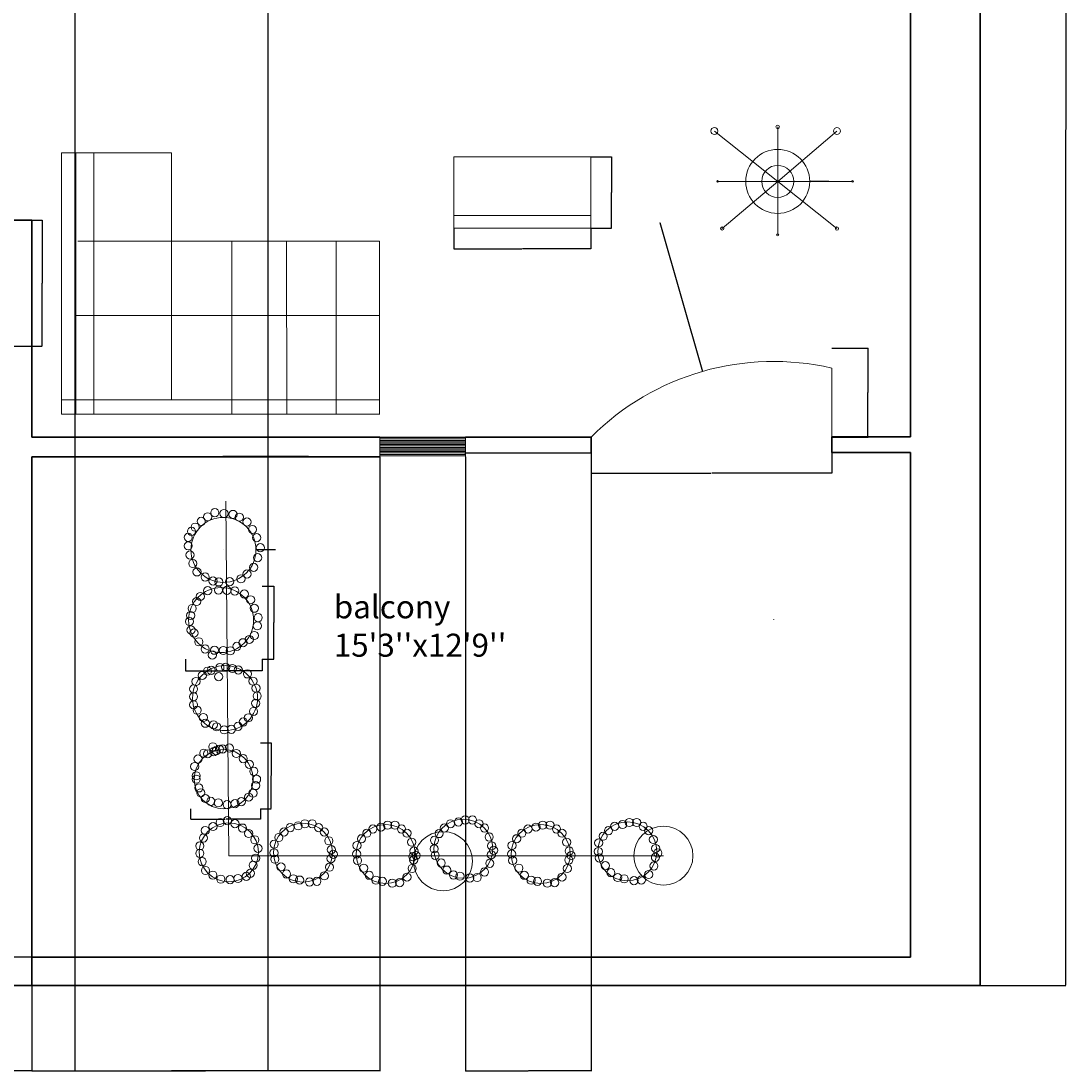
# Model space of a CAD drawing. Units: millimetres. Extents: x 1942 to 12281, y -2698 to 3078.
# Tile 5 of 6: x 9104 to 12281, y -2646 to 547. Entities that reach past the tile are written whole.
import ezdxf

# ---------------------------------------------------------------- set-up
doc = ezdxf.new("R2010")
doc.units = ezdxf.units.MM
for name, color, linetype, lineweight in [('A-ANNO-DIMS', 2, 'Continuous', 18), ('A-AREA-IDEN', 3, 'Continuous', 18), ('A-DOOR', 4, 'Continuous', 18), ('A-FURN', 8, 'Continuous', 18), ('A-GLAZ', 4, 'Continuous', 18), ('A-GLAZ-PATT', 9, 'Continuous', 13), ('A-WALL', 7, 'Continuous', 35), ('E-LITE', 6, 'Continuous', 18), ('L-PLNT', 3, 'Continuous', 13)]:
    doc.layers.add(name, color=color, linetype=linetype, lineweight=lineweight)
doc.styles.get("Standard").update_dxf_attribs({"font": 'arial.ttf'})
doc.dimstyles.get("Standard").update_dxf_attribs({"dimtxt": 0.18, "dimasz": 0.18, "dimexe": 0.18, "dimexo": 0.0625, "dimgap": 0.09, "dimtad": 0, "dimtih": 1, "dimtoh": 1, "dimdec": 4, "dimzin": 0, "dimdsep": 46, "dimtxsty": 'Standard', "dimcen": 0.09, "dimadec": 0, "dimazin": 0, "dimtfac": 1, "dimtdec": 4, "dimtofl": 0, "dimtmove": 0, "dimatfit": 3, "dimfxl": 1, "dimtolj": 1, "dimtzin": 0, "dimarcsym": 0})

# ---------------------------------------------------------------- blocks, each defined once
blk = doc.blocks.new('SOFA-SECTIONAL')
for p, q in [((0, 794.3), (0, 0)), ((0, 794.3), (334.4, 794.3)), ((43.6, 794.3), (43.6, 0)), ((98.1, 794.3), (98.1, 0)), ((334.4, 794.3), (334.4, 43.6)), ((49.7, 525.6), (966.1, 525.6)), ((517.7, 525.6), (517.9, 0)), ((684.1, 525.6), (684.3, 0)), ((834.9, 525.6), (835.1, 0)), ((966.1, 525.6), (966.3, 0)), ((43.6, 299.6), (966.2, 299.6)), ((0, 43.6), (967.4, 43.6)), ((0, 0), (967.4, 0))]:
    blk.add_line(p, q)
blk = doc.blocks.new('SEAT-LIVING')
for p, q in [((0, 38.6), (0, 0)), ((416.9, 0), (416.9, 38.6)), ((0, 0), (416.9, 0))]:
    blk.add_line(p, q)
blk.add_lwpolyline([(0, 217.2), (416.9, 217.2), (416.9, 38.6), (0, 38.6)], close=True)
blk = doc.blocks.new('CHANDELIER-8ARM')
for p, q in [((203.2, 166), (203.2, 331.7)), ((10.7, 319.2), (10.7, 319.2)), ((203.2, 166), (10.7, 319.2)), ((203.2, 166), (383.4, 319.2)), ((203.2, 166), (20.4, 166)), ((203.2, 166), (34.5, 22.7)), ((203.2, 166), (430.7, 166)), ((203.2, 166), (203.2, 3.4)), ((203.2, 166), (383.4, 22.7))]:
    blk.add_line(p, q)
for centre, radius in [((10.7, 319.2), 10.7), ((203.2, 331.7), 5.5), ((383.4, 319.2), 10.2), ((203.2, 166), 97.3), ((203.2, 166), 97.3), ((203.2, 166), 48.7), ((20.4, 166), 2.45), ((430.7, 166), 2.45), ((34.5, 22.7), 4.8), ((203.2, 3.4), 3.36), ((383.4, 22.7), 4.98)]:
    blk.add_circle(centre, radius)
blk = doc.blocks.new('DOOR-ENTRY')
blk.add_line((731.8, 0.7), (731.8, 209.8))
blk.add_arc((555.2, -555.3), 785.2, 77.0012, 134.997)
blk = doc.blocks.new('PLANT-ROUND')
for centre, radius in [((86.1, 183), 12.4), ((106.4, 189), 12.4), ((128.8, 189), 12.4), ((100.7, 101.4), 89.7), ((27.3, 147.6), 12.4), ((43.2, 164.4), 12.4), ((61.8, 177.4), 12.4), ((148.6, 177.4), 12.4), ((165.4, 164.4), 12.4), ((13.3, 127.1), 12.4), ((179.4, 137.3), 12.4), ((12.4, 101), 12.4), ((186.9, 110.3), 12.4), ((193.1, 96.5), 12.4), ((15.2, 81.4), 12.4), ((33.8, 58.1), 12.4), ((181.3, 57.1), 12.4), ((185.9, 83.2), 12.4), ((50.6, 36.6), 12.4), ((71.2, 21.7), 12.4), ((165.4, 31), 12.4), ((90.8, 18), 12.4), ((120.6, 12.4), 12.4), ((143, 14.2), 12.4)]:
    blk.add_circle(centre, radius)
blk = doc.blocks.new('PLANT-ROUND-2')
for centre, radius in [((93.4, 223.1), 12.4), ((121.1, 220.4), 12.4), ((148.7, 217.6), 12.4), ((119.6, 109.8), 98.8), ((52, 196.4), 12.4), ((71.3, 210.2), 12.4), ((168, 209.3), 12.4), ((191, 194.6), 12.4), ((12.4, 147.7), 12.4), ((22.5, 166.1), 12.4), ((33.6, 178.9), 12.4), ((207.6, 171.6), 12.4), ((12.4, 121.9), 12.4), ((220.5, 146.7), 12.4), ((231.6, 116.4), 12.4), ((17.9, 94.3), 12.4), ((223.3, 86), 12.4), ((26.2, 68.5), 12.4), ((211.3, 56.6), 12.4), ((39.1, 42.8), 12.4), ((64, 27.1), 12.4), ((172.6, 21.6), 12.4), ((191, 36.3), 12.4), ((87.9, 15.1), 12.4), ((105.4, 12.4), 12.4), ((138.6, 13.3), 12.4)]:
    blk.add_circle(centre, radius)
blk = doc.blocks.new('PLANT-ROUND-3')
for centre, radius in [((108.8, 118.6), 98.8), ((45.5, 190.7), 12.4), ((67.6, 208.2), 12.4), ((100.8, 210), 12.4), ((126.6, 209.1), 12.4), ((150.5, 207.3), 12.4), ((179.1, 198.1), 12.4), ((198.4, 180.6), 12.4), ((20.7, 153.9), 12.4), ((34.5, 175.1), 12.4), ((209.5, 154.8), 12.4), ((16.1, 132.7), 12.4), ((221.4, 126.3), 12.4), ((12.4, 114.3), 12.4), ((17, 88.6), 12.4), ((218.7, 101.4), 12.4), ((26.2, 79.4), 12.4), ((40.9, 52.7), 12.4), ((194.7, 60), 12.4), ((209.5, 72), 12.4), ((60.1, 30.8), 12.4), ((88.6, 27.1), 12.4), ((115.3, 26.2), 12.4), ((136.5, 25.3), 12.4), ((156.7, 39.1), 12.4), ((175.4, 49.9), 12.4), ((82.2, 12.4), 12.4), ((82.2, 12.4), 12.4), ((82.2, 12.4), 12.4)]:
    blk.add_circle(centre, radius)
blk = doc.blocks.new('PLANT-ROUND-4')
for centre, radius in [((108, 108.9), 98.8), ((54.7, 190.9), 12.4), ((65.8, 193.7), 12.4), ((92.5, 202), 12.4), ((110, 202.9), 12.4), ((130.3, 199.2), 12.4), ((148.7, 194.6), 12.4), ((176.3, 182.6), 12.4), ((19.8, 159.6), 12.4), ((39.1, 178), 12.4), ((88.8, 174.3), 12.4), ((88.8, 174.3), 12.4), ((88.8, 174.3), 12.4), ((88.8, 174.3), 12.4), ((192.9, 160.5), 12.4), ((12.4, 136.6), 12.4), ((202.1, 139.4), 12.4), ((205.8, 115.5), 12.4), ((12.4, 113.6), 12.4), ((12.4, 88.8), 12.4), ((201.2, 93.4), 12.4), ((23.4, 72.2), 12.4), ((194.7, 68.5), 12.4), ((41.9, 50.1), 12.4), ((48.3, 32.6), 12.4), ((73.2, 28), 12.4), ((82.4, 21.6), 12.4), ((147.8, 23.4), 12.4), ((163.4, 36.3), 12.4), ((179.1, 49.2), 12.4), ((105.4, 12.4), 12.4), ((127.5, 14.2), 12.4)]:
    blk.add_circle(centre, radius)
blk = doc.blocks.new('PLANT-ROUND-5')
for centre, radius in [((67.6, 188.1), 12.4), ((87.9, 180.8), 12.4), ((97.1, 181.7), 12.4), ((117.6, 184.4), 12.4), ((22.5, 151.3), 12.4), ((100.5, 89.8), 89.7), ((40, 168.8), 12.4), ((52, 167), 12.4), ((70.4, 173.4), 12.4), ((77.8, 176.2), 12.4), ((138.8, 167.8), 12.4), ((159.9, 152.2), 12.4), ((12.4, 128.3), 12.4), ((178.4, 134.7), 12.4), ((17, 99.8), 12.4), ((17, 89.7), 12.4), ((192.2, 113.5), 12.4), ((200.5, 89.6), 12.4), ((25, 63.2), 12.4), ((25, 63.2), 12.4), ((25, 63.2), 12.4), ((25, 63.2), 12.4), ((25, 63.2), 12.4), ((25, 63.2), 12.4), ((197.7, 70.3), 12.4), ((30.8, 48.3), 12.4), ((44.6, 30.8), 12.4), ((61.2, 22.5), 12.4), ((154.2, 21.6), 12.4), ((176.5, 35.3), 12.4), ((189.4, 47.2), 12.4), ((84.2, 17.9), 12.4), ((110.9, 12.4), 12.4), ((134.9, 15.1), 12.4)]:
    blk.add_circle(centre, radius)
blk = doc.blocks.new('PLANT-ROUND-6')
for centre, radius in [((74, 186.3), 12.4), ((95.8, 192.1), 12.4), ((119.1, 182.8), 12.4), ((100.5, 95.9), 89.7), ((28.8, 162.1), 12.4), ((52.4, 174), 12.4), ((141.9, 169.4), 12.4), ((160.8, 153), 12.4), ((23.3, 139.1), 12.4), ((179.6, 133.8), 12.4), ((12.4, 115.2), 12.4), ((12.4, 92.5), 12.4), ((189.2, 107.7), 12.4), ((19.4, 67.4), 12.4), ((174.3, 56.2), 12.4), ((182.2, 78), 12.4), ((29.6, 40.4), 12.4), ((52, 26.4), 12.4), ((153.8, 22.6), 12.4), ((165.9, 32), 12.4), ((76.3, 14.2), 12.4), ((104.3, 12.4), 12.4), ((128.6, 16.1), 12.4)]:
    blk.add_circle(centre, radius)
blk = doc.blocks.new('WIN-LIVING')
for p, q in [((0, 59.6), (0, 0)), ((0, 59.6), (260.2, 59.6)), ((260.2, 0), (260.2, 59.6))]:
    blk.add_line(p, q)
blk = doc.blocks.new('*D30')
at = {"layer": 'A-ANNO-DIMS', "color": 0, "lineweight": -2, "transparency": 16777216}
for p, q in [((10419.7, -83.7), (10419.7, -146.3)), ((10836.6, -83.7), (10836.6, -146.3)), ((10419.9, -146.2), (10627.2, -146.2)), ((10836.4, -146.2), (10629.1, -146.2))]:
    blk.add_line(p, q, dxfattribs=at)
at = {"layer": 'A-ANNO-DIMS', "color": 0, "transparency": 16777216}
for points in [[(10419.9, -146.1), (10419.9, -146.2), (10419.7, -146.2)], [(10836.4, -146.1), (10836.4, -146.2), (10836.6, -146.2)]]:
    blk.add_solid(points, dxfattribs=at)
at = {"layer": 'Defpoints', "color": 0, "transparency": 16777216}
for p in [(10419.7, -83.6), (10836.6, -83.6), (10836.6, -146.2)]:
    blk.add_point(p, dxfattribs=at)
at = {"layer": 'A-ANNO-DIMS', "color": 0, "transparency": 16777216, "insert": (10628.2, -146.2), "char_height": 0.18, "attachment_point": 5}
blk.add_mtext('\\A1;SEAT 417 TYP.', dxfattribs=at)
blk = doc.blocks.new('*D31')
at = {"layer": 'A-ANNO-DIMS', "color": 0, "lineweight": -2, "transparency": 16777216}
for p, q in [((10836.7, 133.5), (10899.3, 133.5)), ((10899.1, 133.4), (10899.1, 25.1)), ((10899.1, -83.4), (10899.1, 24.8)), ((10836.7, -83.6), (10899.3, -83.6))]:
    blk.add_line(p, q, dxfattribs=at)
at = {"layer": 'A-ANNO-DIMS', "color": 0, "transparency": 16777216}
for points in [[(10899.1, 133.4), (10899.2, 133.4), (10899.1, 133.5)], [(10899.1, -83.4), (10899.2, -83.4), (10899.1, -83.6)]]:
    blk.add_solid(points, dxfattribs=at)
at = {"layer": 'Defpoints', "color": 0, "transparency": 16777216}
for p in [(10836.6, 133.5), (10899.1, 133.5), (10836.6, -83.6)]:
    blk.add_point(p, dxfattribs=at)
at = {"layer": 'A-ANNO-DIMS', "color": 0, "transparency": 16777216, "insert": (10899.1, 25), "char_height": 0.18, "attachment_point": 5}
blk.add_mtext('\\A1;217 TYP.', dxfattribs=at)
blk = doc.blocks.new('*D39')
at = {"layer": 'A-ANNO-DIMS', "color": 0, "lineweight": -2, "transparency": 16777216}
for p, q in [((9071.9, -58.9), (9169.3, -58.9)), ((9169.1, -59), (9169.1, -250.1)), ((9169.1, -441.5), (9169.1, -250.5)), ((9071.9, -441.7), (9169.3, -441.7))]:
    blk.add_line(p, q, dxfattribs=at)
at = {"layer": 'A-ANNO-DIMS', "color": 0, "transparency": 16777216}
for points in [[(9169.1, -59), (9169.1, -59), (9169.1, -58.9)], [(9169.1, -441.5), (9169.1, -441.5), (9169.1, -441.7)]]:
    blk.add_solid(points, dxfattribs=at)
at = {"layer": 'Defpoints', "color": 0, "transparency": 16777216}
for p in [(9071.8, -58.9), (9169.1, -58.9), (9071.8, -441.7)]:
    blk.add_point(p, dxfattribs=at)
at = {"layer": 'A-ANNO-DIMS', "color": 0, "transparency": 16777216, "insert": (9169.1, -250.3), "char_height": 0.18, "attachment_point": 5}
blk.add_mtext('\\A1;383 TYP.', dxfattribs=at)
blk = doc.blocks.new('*D40')
at = {"layer": 'A-ANNO-DIMS', "color": 0, "lineweight": -2, "transparency": 16777216}
for p, q in [((10837.4, -718.5), (10837.4, -828.4)), ((11569.2, -718.5), (11569.2, -828.4)), ((10837.5, -828.2), (11201.8, -828.2)), ((11569, -828.2), (11204.7, -828.2))]:
    blk.add_line(p, q, dxfattribs=at)
at = {"layer": 'A-ANNO-DIMS', "color": 0, "transparency": 16777216}
for points in [[(10837.5, -828.1), (10837.5, -828.2), (10837.4, -828.2)], [(11569, -828.1), (11569, -828.2), (11569.2, -828.2)]]:
    blk.add_solid(points, dxfattribs=at)
at = {"layer": 'Defpoints', "color": 0, "transparency": 16777216}
for p in [(10837.4, -718.4), (11569.2, -718.4), (11569.2, -828.2)]:
    blk.add_point(p, dxfattribs=at)
at = {"layer": 'A-ANNO-DIMS', "color": 0, "transparency": 16777216, "insert": (11203.3, -828.2), "char_height": 0.18, "attachment_point": 5}
blk.add_mtext('\\A1;ENTRY DOOR 732 TYP.', dxfattribs=at)
blk = doc.blocks.new('*D41')
at = {"layer": 'A-ANNO-DIMS', "color": 0, "lineweight": -2, "transparency": 16777216}
for p, q in [((11569.3, -447.7), (11679.2, -447.7)), ((11679, -447.8), (11679, -582.8)), ((11679, -718.2), (11679, -583.2)), ((11569.3, -718.4), (11679.2, -718.4))]:
    blk.add_line(p, q, dxfattribs=at)
at = {"layer": 'A-ANNO-DIMS', "color": 0, "transparency": 16777216}
for points in [[(11678.9, -447.8), (11679, -447.8), (11679, -447.7)], [(11678.9, -718.2), (11679, -718.2), (11679, -718.4)]]:
    blk.add_solid(points, dxfattribs=at)
at = {"layer": 'Defpoints', "color": 0, "transparency": 16777216}
for p in [(11569.2, -447.7), (11679, -447.7), (11569.2, -718.4)]:
    blk.add_point(p, dxfattribs=at)
at = {"layer": 'A-ANNO-DIMS', "color": 0, "transparency": 16777216, "insert": (11679, -583), "char_height": 0.18, "attachment_point": 5}
blk.add_mtext('\\A1;271 TYP.', dxfattribs=at)
blk = doc.blocks.new('*D52')
at = {"layer": 'A-ANNO-DIMS', "color": 0, "lineweight": -2, "transparency": 16777216}
for p, q in [((9604.1, -1393.8), (9604.1, -1429)), ((9837.9, -1393.8), (9837.9, -1429)), ((9604.3, -1428.8), (9719.8, -1428.8)), ((9837.7, -1428.8), (9722.2, -1428.8))]:
    blk.add_line(p, q, dxfattribs=at)
at = {"layer": 'A-ANNO-DIMS', "color": 0, "transparency": 16777216}
for points in [[(9604.3, -1428.8), (9604.3, -1428.8), (9604.1, -1428.8)], [(9837.7, -1428.8), (9837.7, -1428.8), (9837.9, -1428.8)]]:
    blk.add_solid(points, dxfattribs=at)
at = {"layer": 'Defpoints', "color": 0, "transparency": 16777216}
for p in [(9604.1, -1393.7), (9837.9, -1393.7), (9837.9, -1428.8)]:
    blk.add_point(p, dxfattribs=at)
at = {"layer": 'A-ANNO-DIMS', "color": 0, "transparency": 16777216, "insert": (9721, -1428.8), "char_height": 0.18, "attachment_point": 5}
blk.add_mtext('\\A1;PLANT C 234 TYP.', dxfattribs=at)
blk = doc.blocks.new('*D53')
at = {"layer": 'A-ANNO-DIMS', "color": 0, "lineweight": -2, "transparency": 16777216}
for p, q in [((9838, -1171.3), (9873.2, -1171.3)), ((9873, -1171.5), (9873, -1282.3)), ((9873, -1393.5), (9873, -1282.7)), ((9838, -1393.7), (9873.2, -1393.7))]:
    blk.add_line(p, q, dxfattribs=at)
at = {"layer": 'A-ANNO-DIMS', "color": 0, "transparency": 16777216}
for points in [[(9872.9, -1171.5), (9873, -1171.5), (9873, -1171.3)], [(9872.9, -1393.5), (9873, -1393.5), (9873, -1393.7)]]:
    blk.add_solid(points, dxfattribs=at)
at = {"layer": 'Defpoints', "color": 0, "transparency": 16777216}
for p in [(9837.9, -1171.3), (9873, -1171.3), (9837.9, -1393.7)]:
    blk.add_point(p, dxfattribs=at)
at = {"layer": 'A-ANNO-DIMS', "color": 0, "transparency": 16777216, "insert": (9873, -1282.5), "char_height": 0.18, "attachment_point": 5}
blk.add_mtext('\\A1;222 TYP.', dxfattribs=at)
blk = doc.blocks.new('*D56')
at = {"layer": 'A-ANNO-DIMS', "color": 0, "lineweight": -2, "transparency": 16777216}
for p, q in [((9620.1, -1848.4), (9620.1, -1880.5)), ((9833, -1848.4), (9833, -1880.5)), ((9620.3, -1880.3), (9725.4, -1880.3)), ((9832.8, -1880.3), (9727.7, -1880.3))]:
    blk.add_line(p, q, dxfattribs=at)
at = {"layer": 'A-ANNO-DIMS', "color": 0, "transparency": 16777216}
for points in [[(9620.3, -1880.3), (9620.3, -1880.3), (9620.1, -1880.3)], [(9832.8, -1880.3), (9832.8, -1880.3), (9833, -1880.3)]]:
    blk.add_solid(points, dxfattribs=at)
at = {"layer": 'Defpoints', "color": 0, "transparency": 16777216}
for p in [(9620.1, -1848.4), (9833, -1848.4), (9833, -1880.3)]:
    blk.add_point(p, dxfattribs=at)
at = {"layer": 'A-ANNO-DIMS', "color": 0, "transparency": 16777216, "insert": (9726.5, -1880.3), "char_height": 0.18, "attachment_point": 5}
blk.add_mtext('\\A1;PLANT E 213 TYP.', dxfattribs=at)
blk = doc.blocks.new('*D57')
at = {"layer": 'A-ANNO-DIMS', "color": 0, "lineweight": -2, "transparency": 16777216}
for p, q in [((9833, -1647.8), (9865.1, -1647.8)), ((9864.9, -1648), (9864.9, -1747.9)), ((9864.9, -1848.2), (9864.9, -1748.3)), ((9833, -1848.4), (9865.1, -1848.4))]:
    blk.add_line(p, q, dxfattribs=at)
at = {"layer": 'A-ANNO-DIMS', "color": 0, "transparency": 16777216}
for points in [[(9864.9, -1648), (9864.9, -1648), (9864.9, -1647.8)], [(9864.9, -1848.2), (9864.9, -1848.2), (9864.9, -1848.4)]]:
    blk.add_solid(points, dxfattribs=at)
at = {"layer": 'Defpoints', "color": 0, "transparency": 16777216}
for p in [(9833, -1647.8), (9864.9, -1647.8), (9833, -1848.4)]:
    blk.add_point(p, dxfattribs=at)
at = {"layer": 'A-ANNO-DIMS', "color": 0, "transparency": 16777216, "insert": (9864.9, -1748.1), "char_height": 0.18, "attachment_point": 5}
blk.add_mtext('\\A1;201 TYP.', dxfattribs=at)
blk = doc.blocks.new('*D93')
at = {"layer": 'A-ANNO-DIMS', "color": 0, "lineweight": -2, "transparency": 16777216}
for p, q in [((12020.6, 2817.6), (12281, 2817.6)), ((12280.8, 2817.4), (12280.8, 216.2)), ((12280.8, -2385.3), (12280.8, 215.9)), ((12020.6, -2385.5), (12281, -2385.5))]:
    blk.add_line(p, q, dxfattribs=at)
at = {"layer": 'A-ANNO-DIMS', "color": 0, "transparency": 16777216}
for points in [[(12280.7, 2817.4), (12280.8, 2817.4), (12280.8, 2817.6)], [(12280.7, -2385.3), (12280.8, -2385.3), (12280.8, -2385.5)]]:
    blk.add_solid(points, dxfattribs=at)
at = {"layer": 'Defpoints', "color": 0, "transparency": 16777216}
for p in [(12020.6, 2817.6), (12280.8, 2817.6), (12020.6, -2385.5)]:
    blk.add_point(p, dxfattribs=at)
at = {"layer": 'A-ANNO-DIMS', "color": 0, "transparency": 16777216, "insert": (12280.8, 216.1), "char_height": 0.18, "attachment_point": 5}
blk.add_mtext('\\A1;5203', dxfattribs=at)
blk = doc.blocks.new('*D96')
at = {"layer": 'A-ANNO-DIMS', "color": 0, "lineweight": -2, "transparency": 16777216}
for p, q in [((8507.1, -2385.6), (8507.1, -2645.9)), ((9137.2, -2385.6), (9137.2, -2645.9)), ((8507.3, -2645.7), (8821.8, -2645.7)), ((9137, -2645.7), (8822.5, -2645.7))]:
    blk.add_line(p, q, dxfattribs=at)
at = {"layer": 'A-ANNO-DIMS', "color": 0, "transparency": 16777216}
for points in [[(8507.3, -2645.7), (8507.3, -2645.7), (8507.1, -2645.7)], [(9137, -2645.7), (9137, -2645.7), (9137.2, -2645.7)]]:
    blk.add_solid(points, dxfattribs=at)
at = {"layer": 'Defpoints', "color": 0, "transparency": 16777216}
for p in [(8507.1, -2385.5), (9137.2, -2385.5), (9137.2, -2645.7)]:
    blk.add_point(p, dxfattribs=at)
at = {"layer": 'A-ANNO-DIMS', "color": 0, "transparency": 16777216, "insert": (8822.1, -2645.7), "char_height": 0.18, "attachment_point": 5}
blk.add_mtext('\\A1;630.1', dxfattribs=at)
blk = doc.blocks.new('*D103')
at = {"layer": 'A-ANNO-DIMS', "color": 0, "lineweight": -2, "transparency": 16777216}
for p, q in [((9137.2, -778.3), (9137.2, -2645.9)), ((10195.3, -778.3), (10195.3, -2645.9)), ((9137.4, -2645.7), (9665.8, -2645.7)), ((10195.1, -2645.7), (9666.7, -2645.7))]:
    blk.add_line(p, q, dxfattribs=at)
at = {"layer": 'A-ANNO-DIMS', "color": 0, "transparency": 16777216}
for points in [[(9137.4, -2645.7), (9137.4, -2645.7), (9137.2, -2645.7)], [(10195.1, -2645.7), (10195.1, -2645.7), (10195.3, -2645.7)]]:
    blk.add_solid(points, dxfattribs=at)
at = {"layer": 'Defpoints', "color": 0, "transparency": 16777216}
for p in [(9137.2, -778.3), (10195.3, -778.3), (10195.3, -2645.7)]:
    blk.add_point(p, dxfattribs=at)
at = {"layer": 'A-ANNO-DIMS', "color": 0, "transparency": 16777216, "insert": (9666.2, -2645.7), "char_height": 0.18, "attachment_point": 5}
blk.add_mtext('\\A1;1058.1', dxfattribs=at)
blk = doc.blocks.new('*D104')
at = {"layer": 'A-ANNO-DIMS', "color": 0, "lineweight": -2, "transparency": 16777216}
for p, q in [((10455.6, -778.3), (10455.6, -2645.9)), ((10837.4, -766.5), (10837.4, -2645.9)), ((10455.7, -2645.7), (10646.1, -2645.7)), ((10837.2, -2645.7), (10646.9, -2645.7))]:
    blk.add_line(p, q, dxfattribs=at)
at = {"layer": 'A-ANNO-DIMS', "color": 0, "transparency": 16777216}
for points in [[(10455.7, -2645.7), (10455.7, -2645.7), (10455.6, -2645.7)], [(10837.2, -2645.7), (10837.2, -2645.7), (10837.4, -2645.7)]]:
    blk.add_solid(points, dxfattribs=at)
at = {"layer": 'Defpoints', "color": 0, "transparency": 16777216}
for p in [(10455.6, -778.3), (10837.4, -766.5), (10837.4, -2645.7)]:
    blk.add_point(p, dxfattribs=at)
at = {"layer": 'A-ANNO-DIMS', "color": 0, "transparency": 16777216, "insert": (10646.5, -2645.7), "char_height": 0.18, "attachment_point": 5}
blk.add_mtext('\\A1;381.8', dxfattribs=at)
blk = doc.blocks.new('*D109')
at = {"layer": 'A-ANNO-DIMS', "color": 0, "lineweight": -2, "transparency": 16777216}
for p, q in [((9268.3, 1245.3), (9268.3, -2645.9)), ((9854.3, 1173.9), (9854.3, -2645.9)), ((9268.4, -2645.7), (9561, -2645.7)), ((9854.1, -2645.7), (9561.5, -2645.7))]:
    blk.add_line(p, q, dxfattribs=at)
at = {"layer": 'A-ANNO-DIMS', "color": 0, "transparency": 16777216}
for points in [[(9268.4, -2645.7), (9268.4, -2645.7), (9268.3, -2645.7)], [(9854.1, -2645.7), (9854.1, -2645.7), (9854.3, -2645.7)]]:
    blk.add_solid(points, dxfattribs=at)
at = {"layer": 'Defpoints', "color": 0, "transparency": 16777216}
for p in [(9268.3, 1245.4), (9854.3, 1174), (9854.3, -2645.7)]:
    blk.add_point(p, dxfattribs=at)
at = {"layer": 'A-ANNO-DIMS', "color": 0, "transparency": 16777216, "insert": (9561.3, -2645.7), "char_height": 0.18, "attachment_point": 5}
blk.add_mtext('\\A1;586', dxfattribs=at)
blk = doc.blocks.new('*D113')
at = {"layer": 'A-ANNO-DIMS', "color": 0, "lineweight": -2, "transparency": 16777216}
for p, q in [((11807.9, -2299.8), (7068.5, -2299.8)), ((7068.7, -2300), (7068.7, -2342.5)), ((7068.7, -2385.3), (7068.7, -2342.8)), ((12020.5, -2385.5), (7068.5, -2385.5))]:
    blk.add_line(p, q, dxfattribs=at)
at = {"layer": 'A-ANNO-DIMS', "color": 0, "transparency": 16777216}
for points in [[(7068.7, -2300), (7068.8, -2300), (7068.7, -2299.8)], [(7068.7, -2385.3), (7068.8, -2385.3), (7068.7, -2385.5)]]:
    blk.add_solid(points, dxfattribs=at)
at = {"layer": 'Defpoints', "color": 0, "transparency": 16777216}
for p in [(11807.9, -2299.8), (7068.7, -2385.5), (12020.6, -2385.5)]:
    blk.add_point(p, dxfattribs=at)
at = {"layer": 'A-ANNO-DIMS', "color": 0, "transparency": 16777216, "insert": (7068.7, -2342.6), "char_height": 0.18, "attachment_point": 5}
blk.add_mtext('\\A1;85.68', dxfattribs=at)
blk = doc.blocks.new('*D114')
at = {"layer": 'A-ANNO-DIMS', "color": 0, "lineweight": -2, "transparency": 16777216}
for p, q in [((11046.1, -66), (11046.3, -66)), ((11046.3, -66), (11176.1, -518.7)), ((11392.5, -1273.7), (11392.7, -1273.7)), ((11392.6, -1273.8), (11392.6, -1273.6))]:
    blk.add_line(p, q, dxfattribs=at)
at = {"layer": 'A-ANNO-DIMS', "color": 0, "transparency": 16777216}
blk.add_solid([(11176.1, -518.7), (11176.1, -518.7), (11176.2, -518.9)], dxfattribs=at)
at = {"layer": 'Defpoints', "color": 0, "transparency": 16777216}
for p in [(11176.2, -518.9), (11392.6, -1273.7)]:
    blk.add_point(p, dxfattribs=at)
at = {"layer": 'A-ANNO-DIMS', "color": 0, "transparency": 16777216, "insert": (11045.4, -66), "char_height": 0.18, "attachment_point": 5}
blk.add_mtext('\\A1;2X R785.2', dxfattribs=at)
blk = doc.blocks.new('*D120')
at = {"layer": 'A-ANNO-DIMS', "color": 0, "lineweight": -2, "transparency": 16777216}
for p, q in [((11404.7, 58.9), (11404.9, 58.9)), ((11404.8, 58.8), (11404.8, 59)), ((11560.4, 58.9), (11502.2, 58.9))]:
    blk.add_line(p, q, dxfattribs=at)
at = {"layer": 'A-ANNO-DIMS', "color": 0, "transparency": 16777216}
blk.add_solid([(11502.2, 58.9), (11502.2, 58.9), (11502.1, 58.9)], dxfattribs=at)
at = {"layer": 'Defpoints', "color": 0, "transparency": 16777216}
for p in [(11307.5, 58.9), (11502.1, 58.9)]:
    blk.add_point(p, dxfattribs=at)
at = {"layer": 'A-ANNO-DIMS', "color": 0, "transparency": 16777216, "insert": (11561.1, 58.9), "char_height": 0.18, "attachment_point": 5}
blk.add_mtext('\\A1;2X ∅194.6', dxfattribs=at)
blk = doc.blocks.new('*D121')
at = {"layer": 'A-ANNO-DIMS', "color": 0, "lineweight": -2, "transparency": 16777216}
for p, q in [((9719.9, -1061.4), (9720.1, -1061.4)), ((9720, -1061.5), (9720, -1061.3)), ((9878, -1061.4), (9818.9, -1061.4))]:
    blk.add_line(p, q, dxfattribs=at)
at = {"layer": 'A-ANNO-DIMS', "color": 0, "transparency": 16777216}
blk.add_solid([(9818.9, -1061.4), (9818.9, -1061.4), (9818.8, -1061.4)], dxfattribs=at)
at = {"layer": 'Defpoints', "color": 0, "transparency": 16777216}
for p in [(9621.2, -1061.4), (9818.8, -1061.4)]:
    blk.add_point(p, dxfattribs=at)
at = {"layer": 'A-ANNO-DIMS', "color": 0, "transparency": 16777216, "insert": (9878.8, -1061.4), "char_height": 0.18, "attachment_point": 5}
blk.add_mtext('\\A1;6X ∅197.58', dxfattribs=at)

msp = doc.modelspace()

# ---------------------------------------------------------------- hatches: boundary and pattern name
at = {"layer": 'A-GLAZ-PATT'}
h = msp.add_hatch(dxfattribs=at)
h.set_pattern_fill('ANSI31', color=256, scale=1.34183, angle=135, style=0)
h.paths.add_polyline_path([(10195.307, -778.28), (10455.551, -778.28), (10455.551, -718.636), (10195.307, -718.636)])

# ---------------------------------------------------------------- linework, layer by layer
at = {"layer": 'A-WALL'}
for p, q in [((12020.574, -434.479), (12020.574, 2817.617)), ((11807.937, 2543.304), (11807.937, -434.479)), ((9071.789, -58.855), (9137.19, -58.855)), ((9137.19, -718.636), (9137.19, -58.855)), ((11807.937, -434.479), (11807.937, -717.728)), ((12020.574, -434.479), (12020.574, -1168.691)), ((9137.19, -718.636), (9921.708, -718.636)), ((9921.708, -718.636), (9921.708, -718.636)), ((9921.708, -718.636), (10195.307, -718.636)), ((10455.551, -718.636), (10837.366, -718.396)), ((10837.366, -718.396), (10837.366, -766.46)), ((11807.937, -717.728), (11569.199, -717.728)), ((11569.199, -717.728), (11569.199, -765.296)), ((11807.937, -717.728), (11807.937, -717.787)), ((11807.937, -717.728), (11807.937, -717.787)), ((11575.92, -765.296), (11569.199, -765.296)), ((11575.92, -765.296), (11807.937, -765.296)), ((11807.937, -765.296), (11807.937, -1011.187)), ((9137.19, -1768.927), (9137.19, -778.28)), ((9137.19, -778.28), (9921.708, -778.28)), ((9718.134, -777.971), (9978.378, -777.971)), ((9718.134, -777.971), (9978.378, -777.971)), ((9718.134, -777.971), (9978.378, -777.971)), ((9718.134, -777.971), (9978.378, -777.971)), ((9718.134, -777.971), (9978.378, -777.971)), ((9718.134, -777.971), (9978.378, -777.971)), ((9718.134, -777.971), (9978.378, -777.971)), ((9718.134, -777.971), (9978.378, -777.971)), ((10195.307, -778.28), (9921.708, -778.28)), ((10453.538, -766.921), (10837.366, -766.46)), ((11807.937, -1011.187), (11807.937, -1225.48)), ((12020.574, -1225.48), (12020.574, -1099.908)), ((11807.937, -1225.48), (11807.937, -2299.81)), ((12020.574, -1225.48), (12020.574, -2385.489)), ((9137.19, -2385.489), (9137.19, -1768.927)), ((9137.19, -1768.927), (9137.19, -1768.927)), ((9932.14, -2299.81), (9137.19, -2299.81)), ((9932.14, -2299.81), (11807.937, -2299.81)), ((8507.109, -2385.489), (9137.19, -2385.489)), ((9932.14, -2385.489), (9137.19, -2385.489)), ((12020.574, -2385.489), (9932.14, -2385.489))]:
    msp.add_line(p, q, dxfattribs=at)
at = {"layer": 'L-PLNT'}
for p, q in [((9727.024, -913.437), (9736.425, -1991.455)), ((9736.425, -1991.455), (11057.339, -1991.455)), ((11057.339, -1991.455), (11057.339, -1991.455))]:
    msp.add_line(p, q, dxfattribs=at)
for centre, radius in [((11057.339, -1991.455), 89.689), ((10387.48, -2007.896), 89.689), ((10295.447, -1994.059), 12.385)]:
    msp.add_circle(centre, radius, dxfattribs=at)

# ---------------------------------------------------------------- block references
at = {"layer": 'A-DOOR'}
msp.add_blockref('DOOR-ENTRY', (10837.365, -718.396), dxfattribs=at)
at = {"layer": 'A-FURN'}
for name, p in [('SOFA-SECTIONAL', (9227.881, -648.434)), ('SEAT-LIVING', (10419.723, -83.62))]:
    msp.add_blockref(name, p, dxfattribs=at)
at = {"layer": 'A-GLAZ'}
msp.add_blockref('WIN-LIVING', (10195.307, -778.28), dxfattribs=at)
at = {"layer": 'E-LITE'}
msp.add_blockref('CHANDELIER-8ARM', (11201.547, -107.122), dxfattribs=at)
at = {"layer": 'L-PLNT'}
for name, p in [('PLANT-ROUND-2', (9600.4, -1171.242)), ('PLANT-ROUND-3', (9604.084, -1393.729)), ('PLANT-ROUND-4', (9616.635, -1621.186)), ('PLANT-ROUND-5', (9620.107, -1848.379)), ('PLANT-ROUND-6', (9635.748, -2076.696)), ('PLANT-ROUND', (9860.953, -2083.4)), ('PLANT-ROUND', (10348.115, -2071.623)), ('PLANT-ROUND', (10847.063, -2079.474)), ('PLANT-ROUND', (10112.392, -2087.326)), ('PLANT-ROUND', (10583.839, -2087.326))]:
    msp.add_blockref(name, p, dxfattribs=at)

# ---------------------------------------------------------------- texts
at = {"layer": 'A-AREA-IDEN', "insert": (10055.244, -1199.567), "char_height": 70, "attachment_point": 1}
msp.add_mtext("balcony\\P15'3''x12'9''", dxfattribs=at)

# ---------------------------------------------------------------- dimensions: what is measured, and where the dimension line sits
at = {"layer": 'A-ANNO-DIMS'}
for base, p1, p2, override, picture, middle in [((12280.774, 2817.617), (12020.574, -2385.489), (12020.574, 2817.617), {"dimdec": 0, "dimlfac": 1, "dimrnd": 0, "dimzin": 0, "dimdsep": 46, "dimlunit": 2}, '*D93', (12280.774, 216.064)), ((7068.728, -2385.489), (11807.937, -2299.81), (12020.574, -2385.489), {"dimdec": 2, "dimlfac": 1, "dimrnd": 0, "dimzin": 0, "dimdsep": 46, "dimlunit": 2}, '*D113', (7068.728, -2342.65))]:
    dim = msp.add_linear_dim(base=base, p1=p1, p2=p2, angle=90, dimstyle='Standard', override=override, dxfattribs=at)
    dim.commit()
    dim.dimension.update_dxf_attribs({"geometry": picture, "text_midpoint": middle})
for base, p1, p2, override, picture, middle in [((9854.26, -2645.689), (9268.262, 1245.379), (9854.26, 1173.953), {"dimdec": 0, "dimlfac": 1, "dimrnd": 0, "dimzin": 0, "dimdsep": 46, "dimlunit": 2}, '*D109', (9561.261, -2645.689)), ((10195.307, -2645.689), (9137.19, -778.28), (10195.307, -778.28), {"dimdec": 1, "dimlfac": 1, "dimrnd": 0, "dimzin": 0, "dimdsep": 46, "dimlunit": 2}, '*D103', (9666.249, -2645.689)), ((10837.366, -2645.689), (10455.551, -778.28), (10837.366, -766.46), {"dimdec": 1, "dimlfac": 1, "dimrnd": 0, "dimzin": 0, "dimdsep": 46, "dimlunit": 2}, '*D104', (10646.458, -2645.689)), ((9137.19, -2645.689), (8507.109, -2385.489), (9137.19, -2385.489), {"dimdec": 1, "dimlfac": 1, "dimrnd": 0, "dimzin": 0, "dimdsep": 46, "dimlunit": 2}, '*D96', (8822.15, -2645.689))]:
    dim = msp.add_linear_dim(base=base, p1=p1, p2=p2, dimstyle='Standard', override=override, dxfattribs=at)
    dim.commit()
    dim.dimension.update_dxf_attribs({"geometry": picture, "text_midpoint": middle})
for base, p1, p2, picture, middle in [((10899.133, 133.545), (10836.601, -83.62), (10836.601, 133.545), '*D31', (10899.133, 24.962)), ((9169.091, -58.855), (9071.789, -441.726), (9071.789, -58.855), '*D39', (9169.091, -250.291)), ((11678.974, -447.66), (11569.199, -718.396), (11569.199, -447.66), '*D41', (11678.974, -583.028)), ((9872.976, -1171.319), (9837.903, -1393.729), (9837.903, -1171.319), '*D53', (9872.976, -1282.524)), ((9864.883, -1647.845), (9832.956, -1848.379), (9832.956, -1647.845), '*D57', (9864.883, -1748.112))]:
    dim = msp.add_linear_dim(base=base, p1=p1, p2=p2, angle=90, text='<> TYP.', dimstyle='Standard', override={"dimdec": 0, "dimlfac": 1, "dimrnd": 0, "dimzin": 0, "dimdsep": 46, "dimlunit": 2}, dxfattribs=at)
    dim.commit()
    dim.dimension.update_dxf_attribs({"geometry": picture, "text_midpoint": middle})
for p1, p2, text, override, picture, middle in [((11307.468, 58.905), (11502.057, 58.905), '2X <>', {"dimdec": 1, "dimlfac": 1, "dimrnd": 0, "dimzin": 0, "dimdsep": 46, "dimlunit": 2}, '*D120', (11560.433, 58.905)), ((9621.184, -1061.4), (9818.762, -1061.4), '6X <>', {"dimdec": 2, "dimlfac": 1, "dimrnd": 0, "dimzin": 0, "dimdsep": 46, "dimlunit": 2}, '*D121', (9878.035, -1061.4))]:
    dim = msp.add_diameter_dim_2p(p1=p1, p2=p2, text=text, dimstyle='Standard', override=override, dxfattribs=at)
    dim.commit()
    dim.dimension.update_dxf_attribs({"geometry": picture, "text_midpoint": middle, "dimtype": 163})
for base, p1, p2, text, picture, middle in [((10836.601, -146.152), (10419.723, -83.62), (10836.601, -83.62), 'SEAT <> TYP.', '*D30', (10628.162, -146.152)), ((11569.199, -828.171), (10837.366, -718.396), (11569.199, -718.396), 'ENTRY DOOR <> TYP.', '*D40', (11203.282, -828.171)), ((9837.903, -1428.802), (9604.084, -1393.729), (9837.903, -1393.729), 'PLANT C <> TYP.', '*D52', (9720.993, -1428.802)), ((9832.956, -1880.306), (9620.108, -1848.379), (9832.956, -1848.379), 'PLANT E <> TYP.', '*D56', (9726.532, -1880.306))]:
    dim = msp.add_linear_dim(base=base, p1=p1, p2=p2, text=text, dimstyle='Standard', override={"dimdec": 0, "dimlfac": 1, "dimrnd": 0, "dimzin": 0, "dimdsep": 46, "dimlunit": 2}, dxfattribs=at)
    dim.commit()
    dim.dimension.update_dxf_attribs({"geometry": picture, "text_midpoint": middle})
dim = msp.add_radius_dim(center=(11392.577, -1273.665), mpoint=(11176.15, -518.852), text='2X <>', dimstyle='Standard', override={"dimdec": 1, "dimlfac": 1, "dimrnd": 0, "dimzin": 0, "dimdsep": 46, "dimlunit": 2}, dxfattribs=at)
dim.commit()
dim.dimension.update_dxf_attribs({"geometry": '*D114', "text_midpoint": (11045.441, -65.964), "dimtype": 164})

doc.saveas('drawing.dxf')
